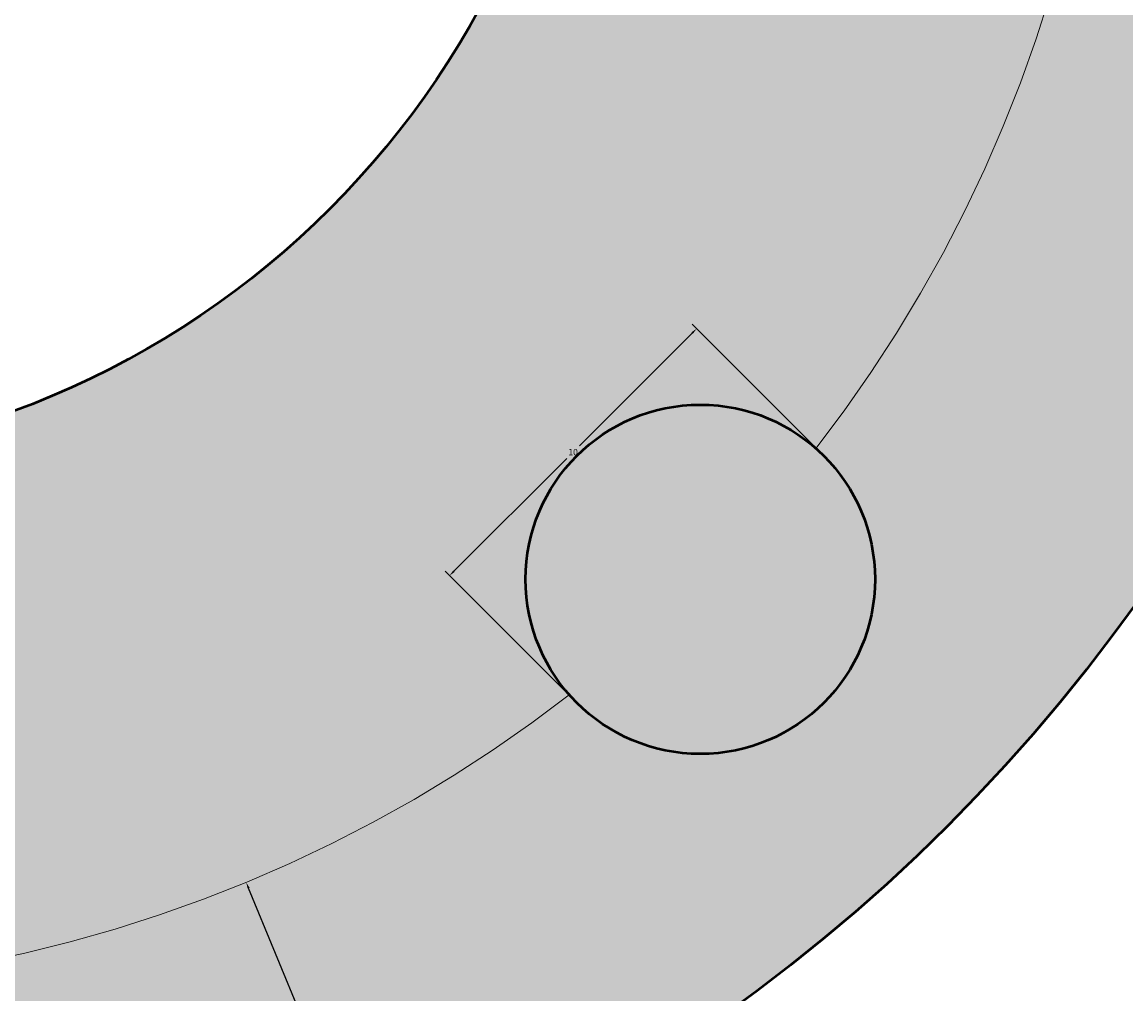
# Model space of a CAD drawing. Units: inches. Extents: x 139261 to 139415, y 52839 to 52963.
# Tile 11 of 20: x 139349 to 139381, y 52860 to 52888. Entities that reach past the tile are written whole.
import ezdxf

# ---------------------------------------------------------------- set-up
doc = ezdxf.new("R2010")
doc.units = ezdxf.units.IN
doc.header["$MEASUREMENT"] = 0
doc.linetypes.add('CENTER', pattern=[50.8, 31.75, -6.35, 6.35, -6.35])
for name, color, linetype, lineweight in [('M-CNTR', 4, 'CENTER', 18), ('M-DIMS', 2, 'Continuous', 25), ('M-HATC', 8, 'Continuous', 18), ('M-OUTL', 7, 'Continuous', 50)]:
    doc.layers.add(name, color=color, linetype=linetype, lineweight=lineweight)
doc.styles.get("Standard").update_dxf_attribs({"font": 'arial.ttf'})
doc.dimstyles.get("Standard").update_dxf_attribs({"dimtxt": 0.18, "dimasz": 0.18, "dimexe": 0.18, "dimexo": 0.0625, "dimgap": 0.09, "dimtad": 0, "dimtih": 1, "dimtoh": 1, "dimdec": 4, "dimzin": 0, "dimdsep": 46, "dimtxsty": 'Standard', "dimcen": 0.09, "dimadec": 0, "dimazin": 0, "dimtfac": 1, "dimtdec": 4, "dimtofl": 0, "dimtmove": 0, "dimatfit": 3, "dimfxl": 1, "dimtolj": 1, "dimtzin": 0, "dimarcsym": 0})

# ---------------------------------------------------------------- blocks, each defined once
blk = doc.blocks.new('*U1')
blk.add_circle((0, 0), 5)
blk = doc.blocks.new('*U2')
at = {"layer": 'M-OUTL', "color": 0, "linetype": 'ByBlock', "lineweight": -2, "transparency": 16777216, "rotation": 225}
blk.add_blockref('*U1', (139368.641, 52871.933), dxfattribs=at)
blk = doc.blocks.new('*D4')
at = {"layer": 'Defpoints', "color": 0, "transparency": 16777216}
for p in [(139373.053, 52923.26), (139307.661, 52877.175)]:
    blk.add_point(p, dxfattribs=at)
at = {"layer": 'M-DIMS', "color": 0, "lineweight": -2, "transparency": 16777216}
for p, q in [((139414.011, 52952.126), (139373.2, 52923.364)), ((139414.191, 52952.126), (139414.011, 52952.126)), ((139340.357, 52900.127), (139340.357, 52900.307)), ((139340.267, 52900.217), (139340.447, 52900.217))]:
    blk.add_line(p, q, dxfattribs=at)
blk.add_arc((139340.357, 52900.217), 40, 34.9168, 52.0771, dxfattribs=at)
at = {"layer": 'M-DIMS', "color": 0, "transparency": 16777216}
blk.add_solid([(139373.183, 52923.388), (139373.217, 52923.339), (139373.053, 52923.26)], dxfattribs=at)
at = {"layer": 'M-DIMS', "color": 0, "transparency": 16777216, "insert": (139414.822, 52952.126), "char_height": 0.18, "attachment_point": 5}
blk.add_mtext('\\A1;∅80.0000', dxfattribs=at)
blk = doc.blocks.new('*D8')
at = {"layer": 'Defpoints', "color": 0, "transparency": 16777216}
for p in [(139368.535, 52879.11), (139372.177, 52875.469), (139365.106, 52868.398)]:
    blk.add_point(p, dxfattribs=at)
at = {"layer": 'M-DIMS', "color": 0, "lineweight": -2, "transparency": 16777216}
for p, q in [((139372.132, 52875.513), (139368.408, 52879.238)), ((139368.408, 52878.983), (139365.181, 52875.757)), ((139361.591, 52872.167), (139364.818, 52875.393)), ((139365.061, 52868.442), (139361.337, 52872.167))]:
    blk.add_line(p, q, dxfattribs=at)
at = {"layer": 'M-DIMS', "color": 0, "transparency": 16777216}
for points in [[(139368.387, 52879.004), (139368.429, 52878.962), (139368.535, 52879.11)], [(139361.57, 52872.188), (139361.613, 52872.145), (139361.464, 52872.039)]]:
    blk.add_solid(points, dxfattribs=at)
at = {"layer": 'M-DIMS', "color": 0, "transparency": 16777216, "insert": (139365, 52875.575), "char_height": 0.18, "attachment_point": 5}
blk.add_mtext('\\A1;10', dxfattribs=at)
blk = doc.blocks.new('*D9')
at = {"layer": 'Defpoints', "color": 0, "transparency": 16777216}
for p in [(139302.054, 52932.357), (139378.659, 52868.078)]:
    blk.add_point(p, dxfattribs=at)
at = {"layer": 'M-DIMS', "color": 0, "lineweight": -2, "transparency": 16777216}
for p, q in [((139278.893, 52951.64), (139279.073, 52951.64)), ((139279.073, 52951.64), (139301.916, 52932.472)), ((139340.357, 52900.127), (139340.357, 52900.307)), ((139340.267, 52900.217), (139340.447, 52900.217))]:
    blk.add_line(p, q, dxfattribs=at)
at = {"layer": 'M-DIMS', "color": 0, "transparency": 16777216}
blk.add_solid([(139301.936, 52932.495), (139301.897, 52932.449), (139302.054, 52932.357)], dxfattribs=at)
at = {"layer": 'M-DIMS', "color": 0, "transparency": 16777216, "insert": (139278.506, 52951.64), "char_height": 0.18, "attachment_point": 5}
blk.add_mtext('\\A1;∅100', dxfattribs=at)
blk = doc.blocks.new('*D10')
at = {"layer": 'Defpoints', "color": 0, "transparency": 16777216}
for p in [(139325.07, 52937.181), (139355.644, 52863.254)]:
    blk.add_point(p, dxfattribs=at)
at = {"layer": 'M-DIMS', "color": 0, "lineweight": -2, "transparency": 16777216}
for p, q in [((139340.357, 52900.127), (139340.357, 52900.307)), ((139340.267, 52900.217), (139340.447, 52900.217)), ((139364.816, 52841.075), (139355.712, 52863.087)), ((139364.996, 52841.075), (139364.816, 52841.075))]:
    blk.add_line(p, q, dxfattribs=at)
at = {"layer": 'M-DIMS', "color": 0, "transparency": 16777216}
blk.add_solid([(139355.74, 52863.099), (139355.685, 52863.076), (139355.644, 52863.254)], dxfattribs=at)
at = {"layer": 'M-DIMS', "color": 0, "transparency": 16777216, "insert": (139365.312, 52841.075), "char_height": 0.18, "attachment_point": 5}
blk.add_mtext('\\A1;∅80', dxfattribs=at)

msp = doc.modelspace()

# ---------------------------------------------------------------- hatches: boundary and pattern name
at = {"layer": 'M-HATC'}
h = msp.add_hatch(color=256, dxfattribs=at)
h.dxf.hatch_style = 1
h.paths.add_polyline_path([(139290.35689, 52900.21749, 1), (139390.35689, 52900.21749, 1)])
h.paths.add_polyline_path([(139335.36666, 52939.90499, -0.01563646), (139335.35689, 52940.21749, -1), (139345.35689, 52940.21749, -0.01563646), (139345.34711, 52939.90499, -0.13461315), (139364.89157, 52931.80941, -0.691035), (139373.64116, 52928.50176, -0.21521822), (139371.94881, 52924.75216, -0.13461315), (139380.04439, 52905.20771, -0.43265224), (139385.35689, 52900.21749, -0.43265224), (139380.04439, 52895.22726, -0.13461315), (139371.94881, 52875.68281, -0.21521822), (139373.64116, 52871.93321, -0.691035), (139364.89157, 52868.62556, -0.13461315), (139345.34711, 52860.52999, -0.01563646), (139345.35689, 52860.21749, -1), (139335.35689, 52860.21749, -0.01563646), (139335.36666, 52860.52999, -0.13461315), (139315.82221, 52868.62556, -0.691035), (139307.07262, 52871.93321, -0.21521822), (139308.76496, 52875.68281, -0.13461315), (139300.66939, 52895.22726, -0.43265224), (139295.35689, 52900.21749, -0.43265224), (139300.66939, 52905.20771, -0.13461315), (139308.76496, 52924.75216, -0.21521822), (139307.07262, 52928.50176, -0.691035), (139315.82221, 52931.80941, -0.13461315)], flags=16)
h.paths.add_polyline_path([(139365.35689, 52900.21749, -1), (139315.35689, 52900.21749, -1)], flags=0)
h.paths.add_polyline_path([(139323.71474, 52911.30978), (139356.99903, 52911.30978, -0.3027197), (139356.99903, 52889.12519), (139323.71474, 52889.12519, -0.3027197)], flags=0)
h.paths.add_polyline_path([(139364.89157, 52931.80941, 0.13461315), (139345.34711, 52939.90499, -0.93933644), (139335.36666, 52939.90499, 0.13461315), (139315.82221, 52931.80941, -0.18270763), (139317.07262, 52928.50176, -0.64579494), (139308.76496, 52924.75216, 0.13461315), (139300.66939, 52905.20771, -0.39601219), (139305.35689, 52900.21749, -0.39601219), (139300.66939, 52895.22726, 0.13461315), (139308.76496, 52875.68281, -0.64579494), (139317.07262, 52871.93321, -0.18270763), (139315.82221, 52868.62556, 0.13461315), (139335.36666, 52860.52999, -0.93933644), (139345.34711, 52860.52999, 0.13461315), (139364.89157, 52868.62556, -0.18270763), (139363.64116, 52871.93321, -0.64579494), (139371.94881, 52875.68281, 0.13461315), (139380.04439, 52895.22726, -0.39601219), (139375.35689, 52900.21749, -0.39601219), (139380.04439, 52905.20771, 0.13461315), (139371.94881, 52924.75216, -0.64579494), (139363.64116, 52928.50176, -0.18270763)], flags=0)
h = msp.add_hatch(color=256, dxfattribs=at)
h.dxf.hatch_style = 1
h.set_gradient(color1=(205, 105, 40), tint=1)
h.paths.add_polyline_path([(139335.35689, 52940.21749, 1), (139345.35689, 52940.21749, 1)])
h.paths.add_polyline_path([(139307.07262, 52928.50176, 1), (139317.07262, 52928.50176, 1)])
h.paths.add_polyline_path([(139295.35689, 52900.21749, 1), (139305.35689, 52900.21749, 1)])
h.paths.add_polyline_path([(139307.07262, 52871.93321, 1), (139317.07262, 52871.93321, 1)])
h.paths.add_polyline_path([(139345.35689, 52860.21749, 1), (139335.35689, 52860.21749, 1)])
h.paths.add_polyline_path([(139363.64116, 52871.93321, 1), (139373.64116, 52871.93321, 1)])
h.paths.add_polyline_path([(139375.35689, 52900.21749, 1), (139385.35689, 52900.21749, 1)])
h.paths.add_polyline_path([(139363.64116, 52928.50176, 1), (139373.64116, 52928.50176, 1)])
h = msp.add_hatch(color=256, dxfattribs=at)
h.dxf.hatch_style = 1
h.paths.add_polyline_path([(139345.34711, 52939.90499, -0.93933644), (139335.36666, 52939.90499, 0.13461315), (139315.82221, 52931.80941, -0.18270763), (139317.07262, 52928.50176, -0.64579494), (139308.76496, 52924.75216, 0.13461315), (139300.66939, 52905.20771, -0.39601219), (139305.35689, 52900.21749, -0.39601219), (139300.66939, 52895.22726, 0.13461315), (139308.76496, 52875.68281, -0.64579494), (139317.07262, 52871.93321, -0.18270763), (139315.82221, 52868.62556, 0.13461315), (139335.36666, 52860.52999, -0.93933644), (139345.34711, 52860.52999, 0.13461315), (139364.89157, 52868.62556, -0.18270763), (139363.64116, 52871.93321, -0.64579494), (139371.94881, 52875.68281, 0.13461315), (139380.04439, 52895.22726, -0.39601219), (139375.35689, 52900.21749, -0.39601219), (139380.04439, 52905.20771, 0.13461315), (139371.94881, 52924.75216, -0.64579494), (139363.64116, 52928.50176, -0.18270763), (139364.89157, 52931.80941, 0.13461315)])
h.paths.add_polyline_path([(139365.35689, 52900.21749, -1), (139315.35689, 52900.21749, -1)], flags=16)
h.paths.add_polyline_path([(139356.99903, 52911.30978, -0.3027197), (139356.99903, 52889.12519), (139323.71474, 52889.12519, -0.3027197), (139323.71474, 52911.30978)], flags=0)

# ---------------------------------------------------------------- linework, layer by layer
at = {"layer": 'M-CNTR'}
for start, end in [(322.166643, 352.833357), (277.166643, 307.833357)]:
    msp.add_arc((139340.35689, 52900.21749), 40, start, end, dxfattribs=at)
at = {"layer": 'M-OUTL'}
for radius in [50, 25]:
    msp.add_circle((139340.35689, 52900.21749), radius, dxfattribs=at)

# ---------------------------------------------------------------- block references
msp.add_blockref('*U2', (0, 0), dxfattribs=at)

# ---------------------------------------------------------------- dimensions: what is measured, and where the dimension line sits
at = {"layer": 'M-DIMS'}
for p1, p2, override, picture, middle in [((139307.66087, 52877.17469), (139373.0529, 52923.26028), {"dimclrd": 0, "dimclre": 0, "dimclrt": 0}, '*D4', (139414.82217, 52952.12585)), ((139378.65939, 52868.07845), (139302.05438, 52932.35652), {"dimdec": 0, "dimlfac": 1, "dimrnd": 0, "dimzin": 0, "dimdsep": 46, "dimlunit": 2}, '*D9', (139278.50641, 52951.63995)), ((139325.07023, 52937.18123), (139355.64354, 52863.25374), {"dimdec": 0, "dimlfac": 1, "dimrnd": 0, "dimzin": 0, "dimdsep": 46, "dimlunit": 2}, '*D10', (139365.31206, 52841.0755))]:
    dim = msp.add_diameter_dim_2p(p1=p1, p2=p2, dimstyle='Standard', override=override, dxfattribs=at)
    dim.commit()
    dim.dimension.update_dxf_attribs({"geometry": picture, "text_midpoint": middle, "dimtype": 163})
dim = msp.add_linear_dim(base=(139368.53509, 52879.11035), p1=(139365.10562, 52868.39768), p2=(139372.17669, 52875.46875), angle=45, dimstyle='Standard', override={"dimdec": 0, "dimlfac": 1, "dimrnd": 0, "dimzin": 0, "dimdsep": 46, "dimlunit": 2}, dxfattribs=at)
dim.commit()
dim.dimension.update_dxf_attribs({"geometry": '*D8', "text_midpoint": (139364.99956, 52875.57481)})

doc.saveas('drawing.dxf')
